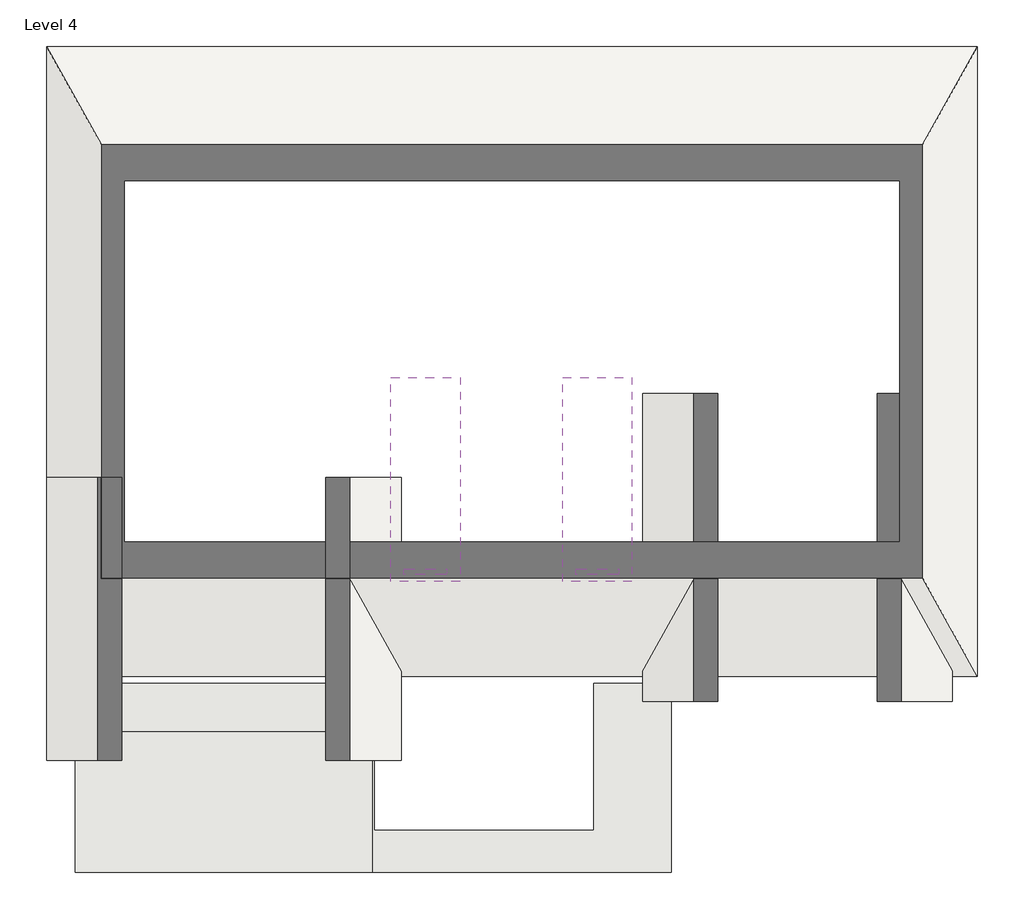
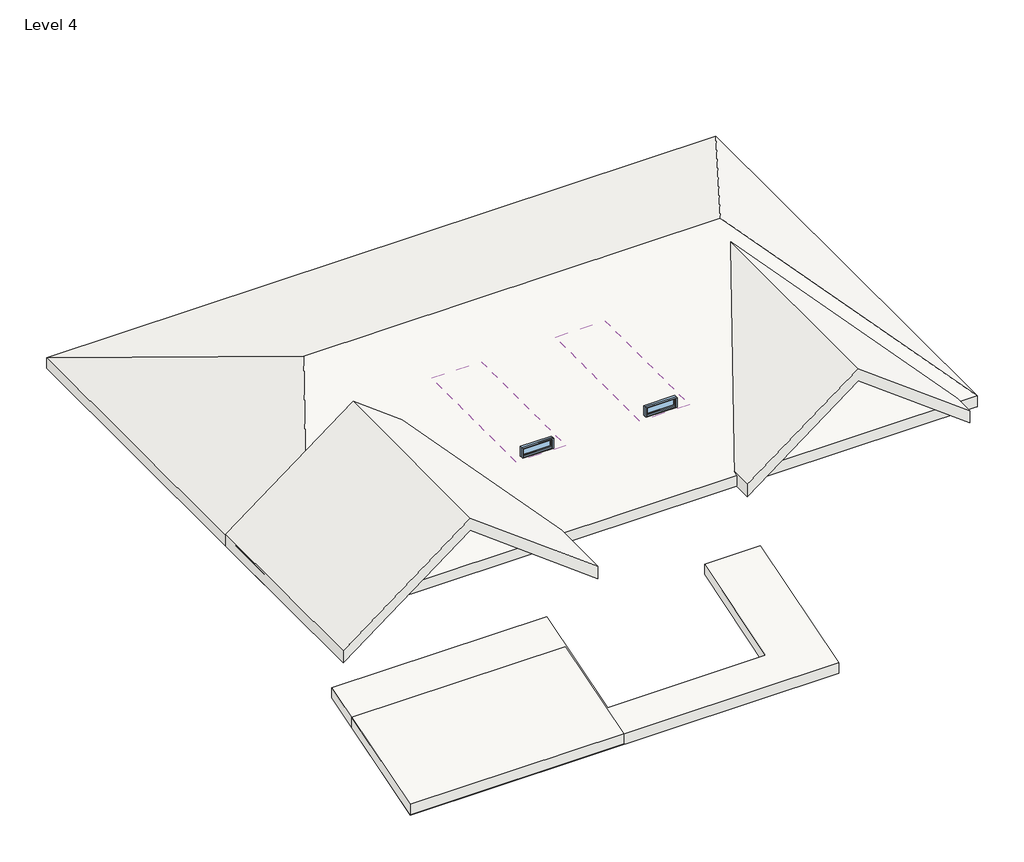
# One storey: 7 roofs, 2 windows.
"""IFC4 building model written with IfcOpenShell, lengths in millimetres."""

from ifc_helpers import new_model, si_unit, frame, origin, place, context, project, spatial, polyline, outline, extrude, faceted_brep, transform, mapped, element, save
from components import fixed_2_x_2_cd9169cd

model = new_model("IFC4")

# Units and contexts
model_context = context("Model", 3, world=origin())
ifc_project = project(units=[si_unit("LENGTHUNIT", "METRE", prefix="MILLI")], contexts=[model_context])

# Site, building, storey
site = spatial("IfcSite", under=ifc_project)
building = spatial("IfcBuilding", under=site)
storey = spatial("IfcBuildingStorey", under=building, Name="Level 4", Elevation=6858.0)

# Roofs
placement = place(None, origin())
element("IfcRoof", 1, ObjectType="Generic - 12\"", at=placement, inside=storey, context=model_context, shape_type="SweptSolid", body=[
    extrude(outline(polyline([(-5372.7787873, 3657.6), (-2381.9111529, 4572.0), (-2381.9111529, 4253.2731526), (-5372.7787873, 3338.8731526), (-5372.7787873, 3657.6)])), frame((-13335.9294011, 0.0, 0.0), z_axis=(1.0, 0.0, 0.0), x_axis=(0.0, 1.0, 0.0)), (0.0, 0.0, 1.0), 6324.6),
])
element("IfcRoof", 2, ObjectType="Generic - 12\"", at=placement, inside=storey, context=model_context, shape_type="Brep", body=[
    faceted_brep([(-648.6294011, -1353.2111529, 4872.5783046), (-648.6294011, -5372.7787873, 3643.6731526), (-648.6294011, -5372.7787873, 3324.9463052), (-648.6294011, -1353.2111529, 4553.8514573), (-13335.9294011, -5372.7787873, 3643.6731526), (-13335.9294011, -1353.2111529, 4872.5783046), (-13335.9294011, -1353.2111529, 4553.8514573), (-13335.9294011, -5372.7787873, 3324.9463052), (-2299.6294011, -1353.2111529, 4872.5783046), (-2299.6294011, -4477.4111529, 3917.4145096), (-6973.2294011, -4477.4111529, 3917.4145096), (-6973.2294011, -1353.2111529, 4872.5783046), (-6973.2294011, -1353.2111529, 4553.8514573), (-6973.2294011, -4477.4111529, 3598.6876622), (-2299.6294011, -4477.4111529, 3598.6876622), (-2299.6294011, -1353.2111529, 4553.8514573)], [[[0, 1, 2, 3]], [[4, 5, 6, 7]], [[1, 0, 8, 9, 10, 11, 5, 4]], [[2, 1, 4, 7]], [[3, 2, 7, 6, 12, 13, 14, 15]], [[0, 3, 15, 8]], [[6, 5, 11, 12]], [[14, 9, 8, 15]], [[10, 13, 12, 11]], [[9, 14, 13, 10]]]),
])
element("IfcRoof", 3, ObjectType="Generic - 12\"", at=placement, inside=storey, context=model_context, shape_type="SweptSolid", body=[
    extrude(outline(polyline([(7239.0, 5333.0705989), (9710.7375, 2037.4205989), (7239.0, -1258.2294011), (6858.0, -1258.2294011), (9329.7375, 2037.4205989), (6858.0, 5333.0705989), (7239.0, 5333.0705989)])), frame((0.0, -1734.2111529, 0.0), z_axis=(0.0, 1.0, 0.0), x_axis=(0.0, 0.0, 1.0)), (0.0, 0.0, 1.0), 6553.2),
])
element("IfcRoof", 4, ObjectType="Generic - 12\"", at=placement, inside=storey, context=model_context, shape_type="Brep", body=[
    faceted_brep([(5798.9479091, 12210.3888471, 6858.0), (2061.5823159, 5504.7888471, 9661.0241949), (-10140.641118, 5504.7888471, 9661.0241949), (-13878.0067113, 12210.3888471, 6858.0), (-13878.0067113, -1200.8111529, 6858.0), (5798.9479091, -1200.8111529, 6858.0), (5866.4705989, 12210.3888471, 7188.3579826), (-13945.5294011, 12210.3888471, 7188.3579826), (-10208.1638079, 5504.7888471, 9991.3821775), (2129.1050057, 5504.7888471, 9991.3821775), (-13945.5294011, -1200.8111529, 7188.3579826), (5866.4705989, -1200.8111529, 7188.3579826), (-13945.5294011, 12210.3888471, 6858.0), (5866.4705989, 12210.3888471, 6858.0), (-13945.5294011, -1200.8111529, 6858.0), (5866.4705989, -1200.8111529, 6858.0)], [[[0, 1, 2, 3]], [[3, 2, 4]], [[1, 0, 5]], [[4, 2, 1, 5]], [[6, 7, 8, 9]], [[7, 10, 8]], [[6, 9, 11]], [[10, 11, 9, 8]], [[12, 7, 6, 13, 0, 3]], [[14, 10, 7, 12]], [[15, 11, 10, 14, 4, 5]], [[13, 6, 11, 15]], [[13, 15, 5, 0]], [[4, 14, 12, 3]]]),
])
element("IfcRoof", 5, ObjectType="Generic - 12\" 2", at=placement, inside=storey, context=model_context, shape_type="SweptSolid", body=[
    extrude(outline(polyline([(7239.0, -6401.7294011), (10067.925, -10173.6294011), (7239.0, -13945.5294011), (6858.0, -13945.5294011), (9686.925, -10173.6294011), (6858.0, -6401.7294011), (7239.0, -6401.7294011)])), frame((0.0, -2991.5111529, 0.0), z_axis=(0.0, 1.0, 0.0), x_axis=(0.0, 0.0, 1.0)), (0.0, 0.0, 1.0), 6019.8),
])
element("IfcRoof", 6, ObjectType="Generic - 12\" 3", at=placement, inside=storey, context=model_context, shape_type="SweptSolid", body=[
    extrude(outline(polyline([(8407.4, -6617.6294011), (8263.7159021, -6617.6294011), (9000.3159021, -5881.0294011), (8263.7159021, -5144.4294011), (8407.4, -5144.4294011), (9144.0, -5881.0294011), (8407.4, -6617.6294011)])), frame((0.0, 823.8671792, 0.0), z_axis=(0.0, 1.0, 0.0), x_axis=(0.0, 0.0, 1.0)), (0.0, 0.0, 1.0), 4338.5470857),
])
element("IfcRoof", 7, ObjectType="Generic - 12\" 3", at=placement, inside=storey, context=model_context, shape_type="SweptSolid", body=[
    extrude(outline(polyline([(8407.4, -2960.0294011), (8263.7159021, -2960.0294011), (9000.3159021, -2223.4294011), (8263.7159021, -1486.8294011), (8407.4, -1486.8294011), (9144.0, -2223.4294011), (8407.4, -2960.0294011)])), frame((0.0, 823.8671792, 0.0), z_axis=(0.0, 1.0, 0.0), x_axis=(0.0, 0.0, 1.0)), (0.0, 0.0, 1.0), 4338.5470857),
])

# Windows
fixed_2_x_2_shape = fixed_2_x_2_cd9169cd(model_context)
element("IfcWindow", 8, ObjectType="Fixed : 2' X 2'", at=placement, inside=storey, context=model_context, shape_type="MappedRepresentation", body=[
    mapped(fixed_2_x_2_shape, transform((-5847.7686248, 1028.0388471, 7888.0954339), x_axis=(1.0, 0.0, 0.0), y_axis=(0.0, 1.0, 0.0), z_axis=(0.0, 0.0, 1.0))),
])
element("IfcWindow", 9, ObjectType="Fixed : 2' X 2'", at=placement, inside=storey, context=model_context, shape_type="MappedRepresentation", body=[
    mapped(fixed_2_x_2_shape, transform((-2190.1686248, 1028.0388471, 7888.0954339), x_axis=(1.0, 0.0, 0.0), y_axis=(0.0, 1.0, 0.0), z_axis=(0.0, 0.0, 1.0))),
])

save(model, "model.ifc")

# Revit data of these elements
# Type "Generic - 12\""
#   Assembly Code = "B1020"
#   Layers, outside or top first: 1' - 0" "ROOF" (function 1)
# Type "Generic - 12\" 2"
#   Assembly Code = "B1020"
#   Layers, outside or top first: 1' - 0" "Gypsum Wall Board" (function 1)
# Type "Generic - 12\" 3"
#   Assembly Code = "B1020"
#   Layers, outside or top first: 0' - 4" no material (function 1)
# Type "Fixed : 2' X 2'"
#   Type Mark = "18"
#   Construction Type Id = "GSP4R"
#   Assembly Code = "B2020100"
#   Analytic Construction = "1/8 in Pilkington single glazing"
#   Visual Light Transmittance = 0.9
#   Solar Heat Gain Coefficient = 0.78
#   Heat Transfer Coefficient (U) = 0.6496 BTU/(h·ft²·°F)
#   Height = 1' - 0"
#   Default Sill Height = 1' - 0"
#   Width = 3' - 0"
#   Window Inset = 0' - 0 3/4"
#   Define Thermal Properties by = 1
#   Glass Pane Material = Glass
#   Sash Material = Sash
#   Wall Closure = (empty or 0)
# Elements 1, 2 (IfcRoof, "Generic - 12\"")
#   built-in parameter 1001710 = 33615
#   Phase Created = New Construction
#   Materials on its faces: "ROOF"
# Element 3 (IfcRoof, "Generic - 12\"")
#   built-in parameter 1001705 = 31.8594 (stored number, unit not read)
#   built-in parameter 1001710 = 33615
#   Phase Created = New Construction
#   Materials on its faces: "ROOF"
# Element 4 (IfcRoof, "Generic - 12\"")
#   built-in parameter 1001705 = 32.7801 (stored number, unit not read)
#   built-in parameter 1001710 = 33615
#   Phase Created = New Construction
#   Materials on its faces: "ROOF"
# Element 5 (IfcRoof, "Generic - 12\" 2")
#   built-in parameter 1001705 = 33.0313 (stored number, unit not read)
#   built-in parameter 1001710 = 33615
#   Phase Created = New Construction
#   Materials on its faces: "Gypsum Wall Board"
# Elements 6, 7 (IfcRoof, "Generic - 12\" 3")
#   built-in parameter 1001710 = 33615
#   Phase Created = New Construction
#   Materials on its faces: "Default Roof"
# Element 8 (IfcWindow, "Fixed : 2' X 2'")
#   Mark = "1"
#   Phase Created = New Construction
#   Materials on its faces: "Sash", "Glass"
# Element 9 (IfcWindow, "Fixed : 2' X 2'")
#   Mark = "2"
#   Phase Created = New Construction
#   Materials on its faces: "Sash", "Glass"
# Materials
#   "ROOF": class "Generic", colour RGB 120 120 120, transparency 0, Cost = 0
#   "Gypsum Wall Board": class "Generic", colour RGB 127 127 127, transparency 0, Description = "Gypsum Wall Board", Cost = 0
#   "Glass": class "Glass", colour RGB 0 128 192, transparency 0.75, Description = "Soda Lime Glass", Cost = 0
#   "Sash": class "Wood", colour RGB 224 178 126, transparency 0, Cost = 0
#   "Default Roof": colour RGB 88 101 114, transparency 0, Cost = 0
